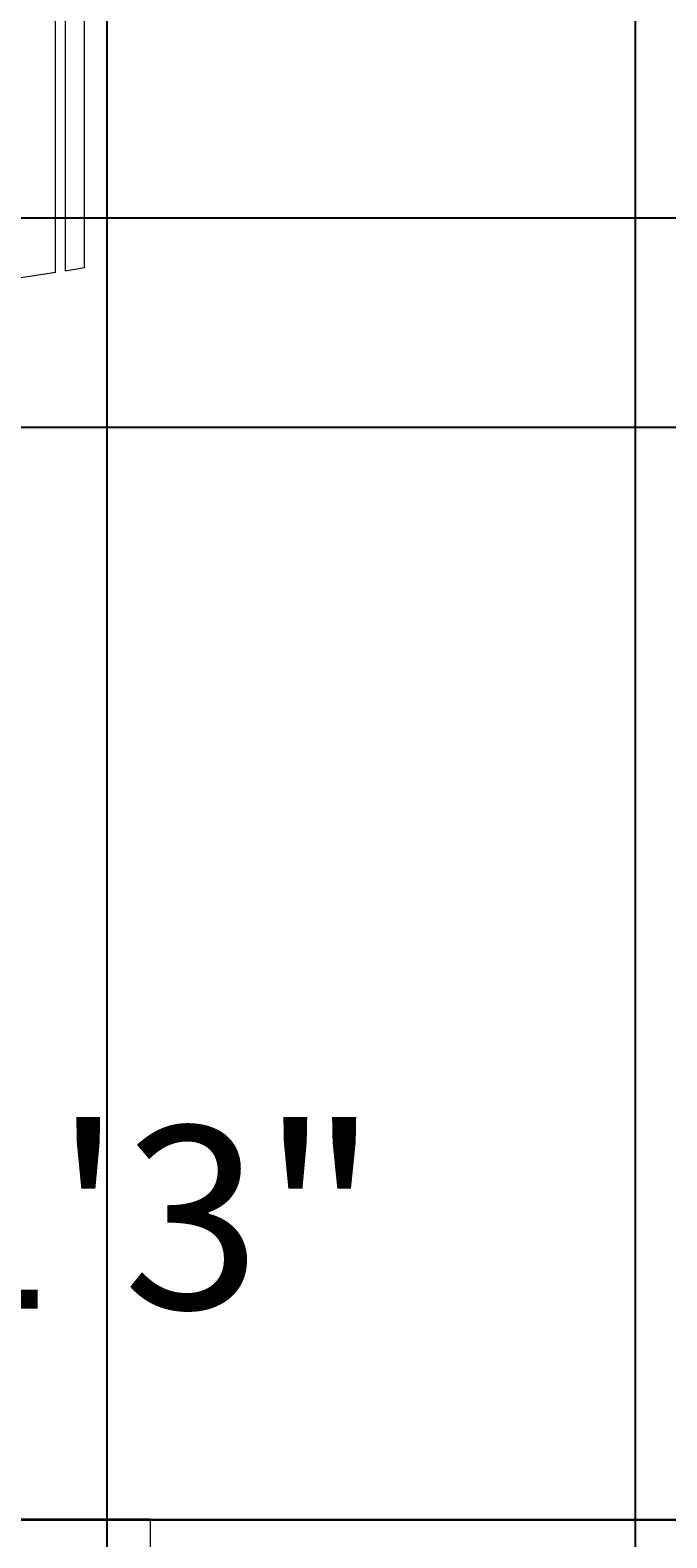
# Model space of a CAD drawing. Units: feet. Extents: x 1654 to 2985, y 1348 to 2230.
# Tile 27 of 53: x 2014 to 2044, y 1750 to 1820. Entities that reach past the tile are written whole.
import ezdxf

# ---------------------------------------------------------------- set-up
doc = ezdxf.new("R2010")
doc.units = ezdxf.units.FT
for name, color, linetype, lineweight in [('A-ANNO-DIMS', 2, 'Continuous', 18), ('A-AREA-IDEN', 7, 'Continuous', 18), ('A-FURN', 8, 'Continuous', 13), ('A-WALL', 7, 'Continuous', 35), ('A-WALL-OPEN', 4, 'Continuous', 18)]:
    doc.layers.add(name, color=color, linetype=linetype, lineweight=lineweight)
doc.styles.get("Standard").update_dxf_attribs({"font": 'arial.ttf'})
doc.dimstyles.get("Standard").update_dxf_attribs({"dimtxt": 0.18, "dimasz": 0.18, "dimexe": 0.18, "dimexo": 0.0625, "dimgap": 0.09, "dimtad": 0, "dimtih": 1, "dimtoh": 1, "dimdec": 4, "dimzin": 0, "dimdsep": 46, "dimtxsty": 'Standard', "dimcen": 0.09, "dimadec": 0, "dimazin": 0, "dimtfac": 1, "dimtdec": 4, "dimtofl": 0, "dimtmove": 0, "dimatfit": 3, "dimfxl": 1, "dimtolj": 1, "dimtzin": 0, "dimarcsym": 0})

# ---------------------------------------------------------------- blocks, each defined once
blk = doc.blocks.new('Dining Set - 36 x 72 in.')
for p, q in [((-22.2343, -26.0006), (-23.4847, -17.99762)), ((-22.2304, -26), (-5.7608, -26)), ((-22, -27.5), (-22.1562, -26.50044)), ((-5.8416, -26.5), (-22.1534, -26.5)), ((-22, -27.5), (-6, -27.5))]:
    blk.add_line(p, q)
blk = doc.blocks.new('OPENING-PUJA')
for p, q in [((0, 9), (0, 0)), ((36, 9), (36, 0)), ((0, 4.5), (36, 4.5))]:
    blk.add_line(p, q)
blk = doc.blocks.new('*D88')
at = {"layer": 'A-ANNO-DIMS', "color": 0, "lineweight": -2, "transparency": 16777216}
for p, q in [((2017.769, 1661.317), (2017.769, 2148.435)), ((2042.08, 1661.317), (2042.08, 2148.435)), ((2017.949, 2148.255), (2029.547, 2148.255)), ((2041.9, 2148.255), (2030.302, 2148.255))]:
    blk.add_line(p, q, dxfattribs=at)
at = {"layer": 'A-ANNO-DIMS', "color": 0, "transparency": 16777216}
for points in [[(2017.949, 2148.285), (2017.949, 2148.225), (2017.769, 2148.255)], [(2041.9, 2148.285), (2041.9, 2148.225), (2042.08, 2148.255)]]:
    blk.add_solid(points, dxfattribs=at)
at = {"layer": 'Defpoints', "color": 0, "transparency": 16777216}
for p in [(2017.769, 2148.255), (2017.769, 1661.255), (2042.08, 1661.255)]:
    blk.add_point(p, dxfattribs=at)
at = {"layer": 'A-ANNO-DIMS', "color": 0, "transparency": 16777216, "insert": (2029.925, 2148.255), "char_height": 0.18, "attachment_point": 5}
blk.add_mtext('\\A1;24.31', dxfattribs=at)
blk = doc.blocks.new('*D91')
at = {"layer": 'A-ANNO-DIMS', "color": 0, "lineweight": -2, "transparency": 16777216}
for p, q in [((1852.155, 1801.468), (2242.272, 1801.468)), ((2242.092, 1801.288), (2242.092, 1776.544)), ((2242.092, 1751.435), (2242.092, 1776.18)), ((1852.155, 1751.255), (2242.272, 1751.255))]:
    blk.add_line(p, q, dxfattribs=at)
at = {"layer": 'A-ANNO-DIMS', "color": 0, "transparency": 16777216}
for points in [[(2242.062, 1801.288), (2242.122, 1801.288), (2242.092, 1801.468)], [(2242.062, 1751.435), (2242.122, 1751.435), (2242.092, 1751.255)]]:
    blk.add_solid(points, dxfattribs=at)
at = {"layer": 'Defpoints', "color": 0, "transparency": 16777216}
for p in [(1852.092, 1801.468), (2242.092, 1801.468), (1852.092, 1751.255)]:
    blk.add_point(p, dxfattribs=at)
at = {"layer": 'A-ANNO-DIMS', "color": 0, "transparency": 16777216, "insert": (2242.092, 1776.362), "char_height": 0.18, "attachment_point": 5}
blk.add_mtext('\\A1;50.21', dxfattribs=at)
blk = doc.blocks.new('*D98')
at = {"layer": 'A-ANNO-DIMS', "color": 0, "lineweight": -2, "transparency": 16777216}
for p, q in [((2061.03, 1811.081), (1811.912, 1811.081)), ((1812.092, 1810.901), (1812.092, 1781.35)), ((1812.092, 1751.435), (1812.092, 1780.986)), ((2061.03, 1751.255), (1811.912, 1751.255))]:
    blk.add_line(p, q, dxfattribs=at)
at = {"layer": 'A-ANNO-DIMS', "color": 0, "transparency": 16777216}
for points in [[(1812.062, 1810.901), (1812.122, 1810.901), (1812.092, 1811.081)], [(1812.062, 1751.435), (1812.122, 1751.435), (1812.092, 1751.255)]]:
    blk.add_solid(points, dxfattribs=at)
at = {"layer": 'Defpoints', "color": 0, "transparency": 16777216}
for p in [(1812.092, 1811.081), (2061.092, 1811.081), (2061.092, 1751.255)]:
    blk.add_point(p, dxfattribs=at)
at = {"layer": 'A-ANNO-DIMS', "color": 0, "transparency": 16777216, "insert": (1812.092, 1781.168), "char_height": 0.18, "attachment_point": 5}
blk.add_mtext('\\A1;59.83', dxfattribs=at)

msp = doc.modelspace()

# ---------------------------------------------------------------- linework, layer by layer
at = {"layer": 'A-WALL'}
msp.add_line((2019.7567, 1751.2549), (1997.0924, 1751.2549), dxfattribs=at)

# ---------------------------------------------------------------- block references
at = {"layer": 'A-FURN', "xscale": 0.8893748792417884, "yscale": 0.8893748792417884, "zscale": 0.8893748792417884, "rotation": 90}
msp.add_blockref('Dining Set - 36 x 72 in.', (1992.2681, 1828.3522), dxfattribs=at)
at = {"layer": 'A-WALL-OPEN'}
msp.add_blockref('OPENING-PUJA', (2019.757, 1742.255), dxfattribs=at)

# ---------------------------------------------------------------- texts
at = {"layer": 'A-AREA-IDEN'}
msp.add_text('8\'8"X11\'3"', height=8.38114, dxfattribs=at).set_placement((1974.793, 1760.9622))

# ---------------------------------------------------------------- dimensions: what is measured, and where the dimension line sits
at = {"layer": 'A-ANNO-DIMS'}
dim = msp.add_linear_dim(base=(2017.7694, 2148.2549), p1=(2042.0798, 1661.2549), p2=(2017.7694, 1661.2549), dimstyle='Standard', override={"dimdec": 2, "dimlfac": 1, "dimrnd": 0, "dimzin": 0, "dimdsep": 46, "dimlunit": 2}, dxfattribs=at)
dim.commit()
dim.dimension.update_dxf_attribs({"geometry": '*D88', "text_midpoint": (2029.9246, 2148.2549)})
for base, p1, p2, picture, middle in [((1812.0924, 1811.0815), (2061.0924, 1751.2549), (2061.0924, 1811.0815), '*D98', (1812.0924, 1781.1682)), ((2242.0924, 1801.4683), (1852.0924, 1751.2549), (1852.0924, 1801.4683), '*D91', (2242.0924, 1776.3616))]:
    dim = msp.add_linear_dim(base=base, p1=p1, p2=p2, angle=90, dimstyle='Standard', override={"dimdec": 2, "dimlfac": 1, "dimrnd": 0, "dimzin": 0, "dimdsep": 46, "dimlunit": 2}, dxfattribs=at)
    dim.commit()
    dim.dimension.update_dxf_attribs({"geometry": picture, "text_midpoint": middle})

doc.saveas('drawing.dxf')
